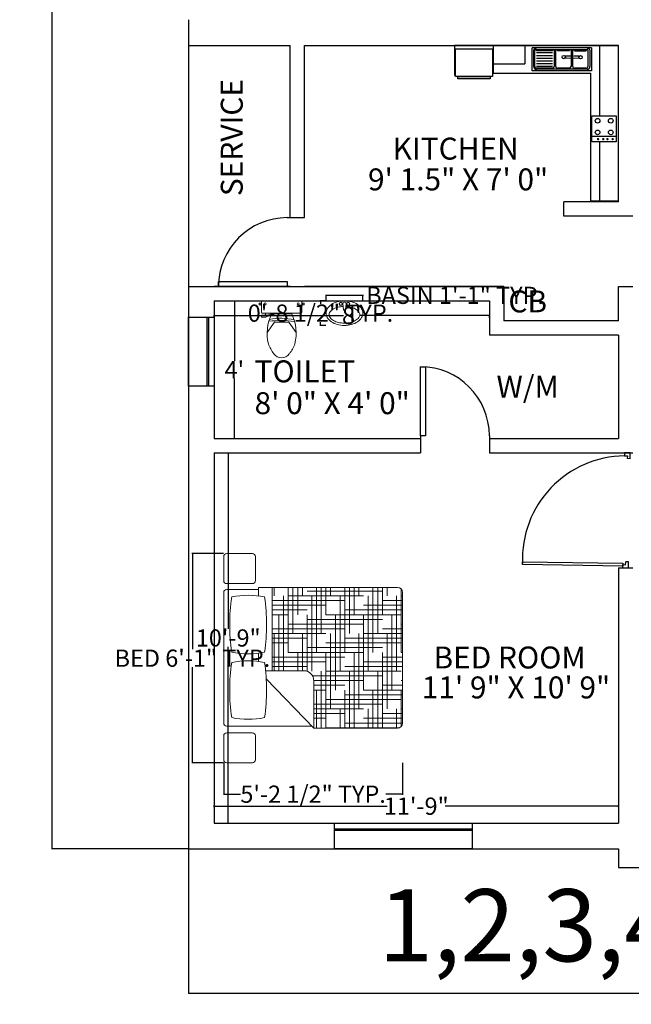
# Model space of a CAD drawing. Units: inches. Extents: x -113 to 5399, y -1393 to 3302.
# Tile 11 of 40: x 1545 to 1759, y 82 to 426. Entities that reach past the tile are written whole.
import ezdxf

# ---------------------------------------------------------------- set-up
doc = ezdxf.new("R2010")
doc.units = ezdxf.units.IN
doc.header["$MEASUREMENT"] = 0
for name, color, linetype, lineweight in [('A-ANNO-DIMS', 254, 'Continuous', 18), ('A-ANNO-TEXT', 7, 'Continuous', 25), ('A-AREA-IDEN', 4, 'Continuous', 18), ('A-FLOR-CASE', 8, 'Continuous', 18), ('A-FLOR-FIXT', 8, 'Continuous', 18), ('doors', 2, 'Continuous', 25), ('DT TEXT', 4, 'Continuous', 18), ('furniture', 131, 'Continuous', 18), ('walls', 1, 'Continuous', 25), ('windows', 3, 'Continuous', 25)]:
    doc.layers.add(name, color=color, linetype=linetype, lineweight=lineweight)
doc.layers.add('A-GLAZ-PATT', color=85, linetype='Continuous', lineweight=13, true_color=0x58ba48)
doc.layers.add('TEFRIŞ', color=11, linetype='Continuous')
doc.styles.get("Standard").update_dxf_attribs({"font": 'arial.ttf'})
doc.dimstyles.get("Standard").update_dxf_attribs({"dimtxt": 6, "dimasz": 0.18, "dimexe": 0.18, "dimexo": 0.0625, "dimgap": 0.09, "dimtad": 0, "dimtih": 1, "dimtoh": 1, "dimdec": 1, "dimzin": 0, "dimdsep": 46, "dimlunit": 4, "dimtxsty": 'Standard', "dimblk": 'ARCHTICK', "dimcen": 0.09, "dimadec": 0, "dimazin": 0, "dimtfac": 1, "dimtdec": 1, "dimtofl": 0, "dimtmove": 0, "dimatfit": 3, "dimfxl": 1, "dimtolj": 1, "dimtzin": 0, "dimarcsym": 0})

# ---------------------------------------------------------------- blocks, each defined once
blk = doc.blocks.new('*U2')
for p, q in [((0, 0), (0, -6)), ((24, 0), (24, -6))]:
    blk.add_line(p, q)
blk.add_lwpolyline([(0, 0), (0, 24), (1.75, 24), (1.75, 0)], close=True)
blk.add_arc((0, 0), 24, 0, 90)
blk = doc.blocks.new('*X4')
at = {"color": 0}
for p, q in [((4.3594, 18.5625), (4.3594, 18.6457)), ((4.5, 18), (4.5, 18.6457)), ((4.5469, 18.1875), (4.5469, 18.6457)), ((4.5938, 18.375), (4.5938, 18.6457)), ((4.6406, 18.5625), (4.6406, 18.6457)), ((4.7812, 18), (4.7812, 18.6457)), ((4.8281, 18.1875), (4.8281, 18.6457)), ((4.875, 18.375), (4.875, 18.6457)), ((4.9219, 18.5625), (4.9219, 18.6457)), ((5.0625, 18), (5.0625, 18.6457)), ((5.1094, 18.1875), (5.1094, 18.6457)), ((5.1562, 18.375), (5.1562, 18.6457)), ((5.2031, 18.5625), (5.2031, 18.6457)), ((5.3438, 18), (5.3438, 18.6457)), ((5.3906, 18.1875), (5.3906, 18.6457)), ((5.4375, 18.375), (5.4375, 18.6457)), ((5.4844, 18.5625), (5.4844, 18.6457)), ((5.625, 18), (5.625, 18.6287)), ((4.4531, 17.8169), (4.4531, 18.5625)), ((4.5, 18.5625), (5.25, 18.5625)), ((4.6875, 18.6094), (5.4375, 18.6094)), ((4.7344, 17.8125), (4.7344, 18.5625)), ((5.0156, 17.8125), (5.0156, 18.5625)), ((5.2969, 17.8125), (5.2969, 18.5625)), ((5.5781, 17.8125), (5.5781, 18.5625)), ((5.625, 18.5625), (5.6375, 18.5625)), ((4.3395, 18.5156), (5.0625, 18.5156)), ((4.3395, 18.4688), (4.875, 18.4688)), ((5.25, 18.4688), (5.6375, 18.4688)), ((5.4375, 18.5156), (5.6375, 18.5156)), ((4.3395, 18.4219), (4.6875, 18.4219)), ((4.3395, 18.375), (4.5, 18.375)), ((4.4062, 17.8169), (4.4062, 18.375)), ((4.6875, 17.8114), (4.6875, 18.375)), ((4.6875, 18.3281), (5.4375, 18.3281)), ((4.875, 18.375), (5.625, 18.375)), ((4.9688, 17.625), (4.9688, 18.375)), ((5.0625, 18.4219), (5.6375, 18.4219)), ((5.25, 17.625), (5.25, 18.375)), ((5.5312, 17.625), (5.5312, 18.375)), ((4.3395, 18.2344), (5.0625, 18.2344)), ((4.5, 18.2812), (5.25, 18.2812)), ((5.4375, 18.2344), (5.6375, 18.2344)), ((5.625, 18.2812), (5.6375, 18.2812)), ((4.3395, 18.1875), (4.875, 18.1875)), ((4.3395, 18.1406), (4.6875, 18.1406)), ((4.3594, 17.8169), (4.3594, 18.1875)), ((4.6406, 17.8169), (4.6406, 18.1875)), ((4.9219, 17.4375), (4.9219, 18.1875)), ((5.0625, 18.1406), (5.6375, 18.1406)), ((5.2031, 17.4375), (5.2031, 18.1875)), ((5.25, 18.1875), (5.6375, 18.1875)), ((5.4844, 17.4375), (5.4844, 18.1875)), ((4.3395, 18.0938), (4.5, 18.0938)), ((4.6875, 18.0469), (5.4375, 18.0469)), ((4.875, 18.0938), (5.625, 18.0938)), ((4.3395, 17.9531), (5.0625, 17.9531)), ((4.5, 18), (5.25, 18)), ((4.5938, 17.8169), (4.5938, 18)), ((4.875, 17.25), (4.875, 18)), ((5.1562, 17.25), (5.1562, 18)), ((5.4375, 17.25), (5.4375, 18)), ((5.4375, 17.9531), (5.6375, 17.9531)), ((5.625, 18), (5.6375, 18)), ((4.3395, 17.9062), (4.875, 17.9062)), ((4.3395, 17.8594), (4.6875, 17.8594)), ((5.0625, 17.8594), (5.6375, 17.8594)), ((5.25, 17.9062), (5.6375, 17.9062)), ((4.7421, 17.7656), (5.4375, 17.7656)), ((4.8281, 17.2457), (4.8281, 17.8125)), ((4.875, 17.8125), (5.625, 17.8125)), ((5.1094, 17.2457), (5.1094, 17.8125)), ((5.3906, 17.2457), (5.3906, 17.8125)), ((4.7548, 17.7188), (5.25, 17.7188)), ((4.7548, 17.6719), (5.0625, 17.6719)), ((5.4375, 17.6719), (5.6375, 17.6719)), ((5.625, 17.7188), (5.6375, 17.7188)), ((4.7548, 17.625), (4.875, 17.625)), ((4.7812, 17.2457), (4.7812, 17.625)), ((5.0625, 17.2457), (5.0625, 17.625)), ((5.0625, 17.5781), (5.6375, 17.5781)), ((5.25, 17.625), (5.6375, 17.625)), ((5.3438, 17.2457), (5.3438, 17.625)), ((5.625, 17.2627), (5.625, 17.625)), ((4.7548, 17.4844), (5.4375, 17.4844)), ((4.875, 17.5312), (5.625, 17.5312)), ((4.7548, 17.4375), (5.25, 17.4375)), ((4.7548, 17.3906), (5.0625, 17.3906)), ((5.0156, 17.2457), (5.0156, 17.4375)), ((5.2969, 17.2457), (5.2969, 17.4375)), ((5.4375, 17.3906), (5.6375, 17.3906)), ((5.5781, 17.2457), (5.5781, 17.4375)), ((5.625, 17.4375), (5.6375, 17.4375)), ((4.7548, 17.3438), (4.875, 17.3438)), ((4.875, 17.25), (5.6077, 17.25)), ((4.9688, 17.2457), (4.9688, 17.25)), ((5.0625, 17.2969), (5.6375, 17.2969)), ((5.25, 17.3438), (5.6375, 17.3438)), ((5.25, 17.2457), (5.25, 17.25)), ((5.5312, 17.2457), (5.5312, 17.25))]:
    blk.add_line(p, q, dxfattribs=at)
blk = doc.blocks.new('MAT-P01')
for p, q in [((-0.0213, 0.8164), (-0.0213, 0.5605)), ((0.0087, 0.8464), (0.2471, 0.8464)), ((0.2771, 0.8164), (0.2771, 0.5605)), ((0.3437, 0.8164), (0.3437, -0.0316)), ((0.3737, 0.8464), (1.6737, 0.8464)), ((1.7037, 0.8164), (1.7037, 0.5005)), ((1.7622, 0.8164), (1.7622, 0.5605)), ((1.7922, 0.8464), (2.0306, 0.8464)), ((2.0606, 0.8164), (2.0606, 0.5605)), ((0.0087, 0.5305), (0.2471, 0.5305)), ((0.9879, 0.5005), (1.0693, 0.5005)), ((1.6393, 0.5005), (1.7237, 0.5005)), ((1.7237, 0.5005), (1.7237, -0.8836)), ((1.7922, 0.5305), (2.0306, 0.5305)), ((0.8146, 0.423), (0.3237, -0.0509)), ((0.8949, 0.4293), (0.8949, 0.0491)), ((0.8949, 0.3643), (1.7237, 0.3643)), ((0.8949, 0.3643), (0.8949, 0.0491)), ((0.8949, 0.3643), (1.7237, 0.3643)), ((1.7237, 0.3643), (1.7237, -0.8836)), ((0.3237, -0.0509), (0.7949, -0.0509)), ((0.3237, -0.0509), (0.3237, -0.8836)), ((0.3737, -0.9336), (1.6737, -0.9336))]:
    blk.add_line(p, q)
for centre, radius, start, end in [((0.0087, 0.8164), 0.03, 90, 180), ((0.2471, 0.8164), 0.03, 0, 90), ((0.3737, 0.8164), 0.03, 90, 180), ((0.7029, -1.1436), 1.9306, 81.81622, 98.18378), ((1.3543, -1.1436), 1.9306, 81.81622, 98.18378), ((1.6737, 0.8164), 0.03, 0, 90), ((1.7922, 0.8164), 0.03, 90, 180), ((2.0306, 0.8164), 0.03, 0, 90), ((1.2251, 0.6034), 0.8138, 168.37298, 191.62702), ((0.1806, 0.6034), 0.8138, 348.37298, 11.62702), ((1.8766, 0.6034), 0.8138, 168.37298, 191.62702), ((0.8321, 0.6034), 0.8138, 348.37298, 11.62702), ((0.0087, 0.5605), 0.03, 180, 270), ((0.2471, 0.5605), 0.03, 270, 0), ((1.7922, 0.5605), 0.03, 180, 270), ((2.0306, 0.5605), 0.03, 270, 0), ((0.7029, 2.3504), 1.9306, 261.81622, 278.18378), ((1.3543, 2.3504), 1.9306, 261.81622, 278.18378), ((0.7949, 0.0491), 0.1, 270, 0), ((0.3737, -0.8836), 0.05, 180, 270), ((1.6737, -0.8836), 0.05, 270, 0)]:
    blk.add_arc(centre, radius, start, end)
at = {"rotation": 270}
blk.add_blockref('*X4', (-16.9221, 4.7038), dxfattribs=at)
blk = doc.blocks.new('A$C008029BD')
at = {"layer": 'TEFRIŞ', "ltscale": 0.05}
for p, q in [((0, 0), (0, -3.55)), ((3.37, 0), (0, 0)), ((3.37, 0), (3.37, -0.6)), ((1.522, -0.4), (0, -0.4)), ((3.37, -0.4), (2.083, -0.4)), ((0.05, -0.581), (0.05, -1.869)), ((0.05, -0.581), (0.55, -0.581)), ((0.096, -0.617), (0.454, -0.617)), ((0.55, -0.581), (0.55, -1.869)), ((0.6, -2.71), (0.6, -0.6)), ((3.37, -0.6), (0.6, -0.6)), ((0.086, -1.773), (0.086, -0.677)), ((0.099, -0.659), (0.457, -0.659)), ((0.113, -0.954), (0.113, -0.695)), ((0.23, -0.846), (0.229, -0.967)), ((0.28, -0.846), (0.277, -1.158)), ((0.493, -0.695), (0.493, -0.954)), ((0.514, -0.677), (0.514, -1.773)), ((0.096, -1.024), (0.454, -1.024)), ((0.457, -0.99), (0.099, -0.99)), ((0.11, -1.319), (0.11, -1.06)), ((0.228, -1.02), (0.227, -1.159)), ((0.49, -1.06), (0.49, -1.319)), ((0.454, -1.355), (0.096, -1.355)), ((0.096, -1.391), (0.454, -1.391)), ((0.11, -1.773), (0.11, -1.427)), ((0.154, -1.773), (0.154, -1.427)), ((0.214, -1.773), (0.214, -1.427)), ((0.274, -1.773), (0.274, -1.427)), ((0.334, -1.773), (0.334, -1.427)), ((0.39, -1.773), (0.39, -1.427)), ((0.444, -1.773), (0.444, -1.427)), ((0.49, -1.427), (0.49, -1.773)), ((0.55, -1.869), (0.05, -1.869)), ((0.454, -1.809), (0.096, -1.809)), ((0.454, -1.833), (0.096, -1.833)), ((0, -2.025), (0.4, -2.025)), ((0.4, -2.71), (0.4, -2.025)), ((0, -2.71), (0.6, -2.71)), ((0, -3.55), (0.65, -3.55))]:
    blk.add_line(p, q, dxfattribs=at)
at = {"layer": 'TEFRIŞ'}
blk.add_line((1.969, -0.05), (1.969, -0.572), dxfattribs=at)
at = {"layer": 'TEFRIŞ', "ltscale": 0.05}
for points in [[(1.522, -0.05), (2.083, -0.05), (2.083, -0.572), (1.522, -0.572)], [(0.67, -2.73), (0.67, -3.53), (0.07, -3.53), (0.07, -2.73)], [(0.72, -2.78), (0.72, -3.48), (0.67, -3.48), (0.67, -2.78)]]:
    blk.add_lwpolyline(points, close=True, dxfattribs=at)
at = {"layer": 'TEFRIŞ', "const_width": 0.025}
for points in [[(2.014, -0.123, 1), (2.039, -0.123, 1)], [(2.014, -0.236, 1), (2.039, -0.236, 1)], [(2.014, -0.327, 1), (2.039, -0.327, 1)], [(2.014, -0.44, 1), (2.039, -0.44, 1)]]:
    blk.add_lwpolyline(points, format="xyb", close=True, dxfattribs=at)
at = {"layer": 'TEFRIŞ', "ltscale": 0.05}
for centre, radius in [((1.628, -0.164), 0.0505), ((1.628, -0.45), 0.0505), ((0.255, -0.82), 0.036), ((0.252, -1.184), 0.036)]:
    blk.add_circle(centre, radius, dxfattribs=at)
at = {"layer": 'TEFRIŞ'}
for centre in [(1.88, -0.164), (1.88, -0.45)]:
    blk.add_circle(centre, 0.0505, dxfattribs=at)
at = {"layer": 'TEFRIŞ', "ltscale": 0.05}
for centre, radius, start, end in [((0.108, -0.649), 0.0351, 110.4976, 230.5777), ((0.454, -0.677), 0.06, 0, 90), ((0.118, -0.673), 0.023, 143.9853, 258.5157), ((0.457, -0.695), 0.036, 0, 90), ((0.115, -1.038), 0.023, 143.9853, 258.5157), ((0.118, -0.976), 0.023, 101.4843, 216.0147), ((0.454, -1.06), 0.036, 0, 90), ((0.457, -0.954), 0.036, 270, 0), ((0.115, -1.341), 0.023, 101.4843, 216.0147), ((0.115, -1.405), 0.023, 143.9853, 258.5157), ((0.454, -1.319), 0.036, 270, 0), ((0.454, -1.427), 0.036, 0, 90), ((0.108, -1.801), 0.0351, 129.4223, 249.5024), ((0.115, -1.796), 0.023, 101.4843, 216.0147), ((0.454, -1.773), 0.06, 270, 0), ((0.454, -1.773), 0.036, 270, 0)]:
    blk.add_arc(centre, radius, start, end, dxfattribs=at)
blk = doc.blocks.new('toilet-3')
at = {"color": 0, "linetype": 'ByBlock'}
for p, q in [((-0.281, -0.05), (-0.281, -0.069)), ((-0.281, -0.05), (-0.261, -0.05)), ((-0.281, -0.069), (-0.261, -0.069)), ((-0.261, -0.047), (-0.261, -0.072)), ((-0.261, -0.047), (-0.251, -0.047)), ((-0.261, -0.072), (-0.251, -0.072)), ((-0.251, -0.047), (-0.251, -0.072)), ((-0.25, -0.03), (-0.25, -0.165)), ((0.24, -0.02), (-0.24, -0.02)), ((0.25, -0.03), (0.25, -0.165)), ((0.261, -0.047), (0.251, -0.047)), ((0.251, -0.047), (0.251, -0.072)), ((0.261, -0.072), (0.251, -0.072)), ((0.261, -0.047), (0.261, -0.072)), ((0.281, -0.05), (0.261, -0.05)), ((0.281, -0.069), (0.261, -0.069)), ((0.281, -0.05), (0.281, -0.069)), ((-0.144, -0.2), (-0.25, -0.2)), ((-0.25, -0.2), (-0.25, -0.222)), ((-0.198, -0.222), (-0.25, -0.222)), ((0.24, -0.175), (-0.24, -0.175)), ((-0.202, -0.2), (-0.202, -0.175)), ((-0.198, -0.222), (-0.16, -0.207)), ((-0.16, -0.207), (-0.16, -0.2)), ((-0.144, -0.2), (-0.144, -0.175)), ((0.125, -0.182), (-0.125, -0.182)), ((-0.089, -0.287), (-0.18, -0.415)), ((0.089, -0.287), (-0.089, -0.287)), ((0.089, -0.287), (0.18, -0.415))]:
    blk.add_line(p, q, dxfattribs=at)
for centre in [(-0.205, -0.059), (0.205, -0.059)]:
    blk.add_circle(centre, 0.0125, dxfattribs=at)
for centre, radius, start, end in [((-0.24, -0.03), 0.01, 90, 180), ((0.24, -0.03), 0.01, 0, 90), ((-0.24, -0.165), 0.01, 180, 270), ((0.376, -0.424), 0.557, 154.2321, 193.6755), ((-0.005, -0.896), 0.659, 75.9276, 103.0204), ((-0.376, -0.424), 0.557, 346.3245, 25.7679), ((0.24, -0.165), 0.01, 270, 0), ((-0.013, -1.787), 1.521, 83.4552, 95.5271), ((0.262, -0.406), 0.452, 199.2942, 217.2549), ((-0.265, -0.4), 0.457, 322.2382, 340.1051), ((-0.001, -0.609), 0.12, 216.3794, 323.6206)]:
    blk.add_arc(centre, radius, start, end, dxfattribs=at)
blk = doc.blocks.new('wash-6')
at = {"color": 0, "linetype": 'ByBlock'}
for p, q in [((-0.036, -0.063), (-0.021, -0.18)), ((0.036, -0.063), (0.021, -0.18))]:
    blk.add_line(p, q, dxfattribs=at)
for centre, radius in [((-0.075, -0.062), 0.0325), ((-0.075, -0.062), 0.0263), ((0.075, -0.062), 0.0325), ((0.075, -0.062), 0.0263)]:
    blk.add_circle(centre, radius, dxfattribs=at)
for centre, radius, start, end in [((0, -0.56), 0.56, 90, 105.4371), ((-0.204, -0.25), 0.17, 148.1465, 180), ((-0.107, -0.311), 0.285, 123.6901, 148.1465), ((-0.114, -0.361), 0.225, 118.369, 142.5096), ((-0.042, -0.407), 0.401, 105.4371, 123.6901), ((-0.045, -0.488), 0.37, 102.6081, 118.369), ((0, -0.69), 0.576, 92.9466, 102.6081), ((0, -0.063), 0.0361, 0, 180), ((0, -0.18), 0.0215, 180, 0), ((0, -0.56), 0.56, 74.5629, 90), ((0, -0.69), 0.576, 77.3919, 87.0534), ((0.045, -0.488), 0.37, 61.631, 77.3919), ((0.042, -0.407), 0.401, 56.3099, 74.5629), ((0.114, -0.361), 0.225, 37.4904, 61.631), ((0.107, -0.311), 0.285, 31.8535, 56.3099), ((0.204, -0.25), 0.17, 0, 31.8535), ((-0.204, -0.25), 0.17, 180, 211.8535), ((-0.107, -0.189), 0.285, 211.8535, 236.3099), ((-0.217, -0.282), 0.0954, 142.5096, 180), ((-0.217, -0.282), 0.0954, 180, 217.4904), ((-0.114, -0.203), 0.225, 217.4904, 241.631), ((0.114, -0.203), 0.225, 298.369, 322.5096), ((0.107, -0.189), 0.285, 303.6901, 328.1465), ((0.217, -0.282), 0.0954, 0, 37.4904), ((0.217, -0.282), 0.0954, 322.5096, 0), ((0.204, -0.25), 0.17, 328.1465, 0), ((-0.042, -0.092), 0.401, 236.3099, 254.5629), ((-0.045, -0.076), 0.37, 241.631, 257.3919), ((0, 0.06), 0.56, 254.5629, 270), ((0, 0.125), 0.576, 257.3919, 270), ((0, 0.125), 0.576, 270, 282.6081), ((0, 0.06), 0.56, 270, 285.4371), ((0.045, -0.076), 0.37, 282.6081, 298.369), ((0.042, -0.092), 0.401, 285.4371, 303.6901)]:
    blk.add_arc(centre, radius, start, end, dxfattribs=at)
blk = doc.blocks.new('_ArchTick')
at = {"color": 0, "linetype": 'ByBlock', "const_width": 0.15}
blk.add_lwpolyline([(-0.5, -0.5), (0.5, 0.5)], dxfattribs=at)
blk = doc.blocks.new('*D59')
at = {"layer": 'A-ANNO-DIMS', "color": 0, "lineweight": -2, "transparency": 16777216}
for p, q in [((1604.26, 136.47), (1604.26, 86.09)), ((2037.26, 136.47), (2037.26, 86.09)), ((1604.26, 86.27), (1810.37, 86.27)), ((2037.26, 86.27), (1831.16, 86.27))]:
    blk.add_line(p, q, dxfattribs=at)
at = {"layer": 'Defpoints', "color": 0, "transparency": 16777216}
for p in [(1604.26, 136.53), (2037.26, 136.53), (2037.26, 86.27)]:
    blk.add_point(p, dxfattribs=at)
at = {"layer": 'A-ANNO-DIMS', "color": 0, "lineweight": -2, "transparency": 16777216, "xscale": 0.18, "yscale": 0.18, "zscale": 0.18, "rotation": 180}
blk.add_blockref('_ArchTick', (1604.26, 86.27), dxfattribs=at)
at = {"layer": 'A-ANNO-DIMS', "color": 0, "lineweight": -2, "transparency": 16777216, "xscale": 0.18, "yscale": 0.18, "zscale": 0.18}
blk.add_blockref('_ArchTick', (2037.26, 86.27), dxfattribs=at)
at = {"layer": 'A-ANNO-DIMS', "color": 0, "transparency": 16777216, "insert": (1820.76, 86.27), "char_height": 6, "attachment_point": 5}
blk.add_mtext('\\A1;36\'-1"', dxfattribs=at)
blk = doc.blocks.new('*D60')
at = {"layer": 'A-ANNO-DIMS', "color": 0, "lineweight": -2, "transparency": 16777216}
for p, q in [((1604.2, 786.53), (1556.55, 786.53)), ((1556.73, 786.53), (1556.73, 464.69)), ((1556.73, 136.53), (1556.73, 458.38)), ((1604.2, 136.53), (1556.55, 136.53))]:
    blk.add_line(p, q, dxfattribs=at)
at = {"layer": 'Defpoints', "color": 0, "transparency": 16777216}
for p in [(1604.26, 786.53), (1556.73, 136.53), (1604.26, 136.53)]:
    blk.add_point(p, dxfattribs=at)
at = {"layer": 'A-ANNO-DIMS', "color": 0, "lineweight": -2, "transparency": 16777216, "xscale": 0.18, "yscale": 0.18, "zscale": 0.18}
for p, rotation in [((1556.73, 786.53), 90), ((1556.73, 136.53), 270)]:
    blk.add_blockref('_ArchTick', p, dxfattribs=dict(at, rotation=rotation))
at = {"layer": 'A-ANNO-DIMS', "color": 0, "transparency": 16777216, "insert": (1556.73, 461.53), "char_height": 6, "attachment_point": 5}
blk.add_mtext('\\A1;54\'-2"', dxfattribs=at)
blk = doc.blocks.new('*D67')
at = {"layer": 'A-ANNO-DIMS', "color": 0, "lineweight": -2, "transparency": 16777216}
for p, q in [((1617.62, 274.53), (1618.35, 274.53)), ((1618.17, 274.53), (1618.17, 213.19)), ((1618.17, 145.53), (1618.17, 206.88)), ((1617.62, 145.53), (1618.35, 145.53))]:
    blk.add_line(p, q, dxfattribs=at)
at = {"layer": 'Defpoints', "color": 0, "transparency": 16777216}
for p in [(1617.55, 274.53), (1617.55, 145.53), (1618.17, 145.53)]:
    blk.add_point(p, dxfattribs=at)
at = {"layer": 'A-ANNO-DIMS', "color": 0, "lineweight": -2, "transparency": 16777216, "xscale": 0.18, "yscale": 0.18, "zscale": 0.18}
for p, rotation in [((1618.17, 274.53), 90), ((1618.17, 145.53), 270)]:
    blk.add_blockref('_ArchTick', p, dxfattribs=dict(at, rotation=rotation))
at = {"layer": 'A-ANNO-DIMS', "color": 0, "transparency": 16777216, "insert": (1618.17, 210.03), "char_height": 6, "attachment_point": 5}
blk.add_mtext('\\A1;10\'-9"', dxfattribs=at)
blk = doc.blocks.new('*D68')
at = {"layer": 'A-ANNO-DIMS', "color": 0, "lineweight": -2, "transparency": 16777216}
for p, q in [((1613.26, 151.05), (1613.26, 151.58)), ((1613.26, 151.4), (1673.65, 151.4)), ((1754.26, 151.4), (1693.88, 151.4)), ((1754.26, 151.05), (1754.26, 151.58))]:
    blk.add_line(p, q, dxfattribs=at)
at = {"layer": 'Defpoints', "color": 0, "transparency": 16777216}
for p in [(1754.26, 151.4), (1613.26, 150.98), (1754.26, 150.98)]:
    blk.add_point(p, dxfattribs=at)
at = {"layer": 'A-ANNO-DIMS', "color": 0, "lineweight": -2, "transparency": 16777216, "xscale": 0.18, "yscale": 0.18, "zscale": 0.18, "rotation": 180}
blk.add_blockref('_ArchTick', (1613.26, 151.4), dxfattribs=at)
at = {"layer": 'A-ANNO-DIMS', "color": 0, "lineweight": -2, "transparency": 16777216, "xscale": 0.18, "yscale": 0.18, "zscale": 0.18}
blk.add_blockref('_ArchTick', (1754.26, 151.4), dxfattribs=at)
at = {"layer": 'A-ANNO-DIMS', "color": 0, "transparency": 16777216, "insert": (1683.76, 151.4), "char_height": 6, "attachment_point": 5}
blk.add_mtext('\\A1;11\'-9"', dxfattribs=at)
blk = doc.blocks.new('*D77')
at = {"layer": 'A-ANNO-DIMS', "color": 0, "lineweight": -2, "transparency": 16777216}
for p, q in [((1620.3, 327.53), (1620.3, 306.62)), ((1620.36, 327.53), (1620.48, 327.53)), ((1620.3, 279.53), (1620.3, 300.44)), ((1620.36, 279.53), (1620.48, 279.53))]:
    blk.add_line(p, q, dxfattribs=at)
at = {"layer": 'Defpoints', "color": 0, "transparency": 16777216}
for p in [(1620.3, 327.53), (1620.3, 279.53), (1620.3, 279.53)]:
    blk.add_point(p, dxfattribs=at)
at = {"layer": 'A-ANNO-DIMS', "color": 0, "lineweight": -2, "transparency": 16777216, "xscale": 0.18, "yscale": 0.18, "zscale": 0.18}
for p, rotation in [((1620.3, 327.53), 90), ((1620.3, 279.53), 270)]:
    blk.add_blockref('_ArchTick', p, dxfattribs=dict(at, rotation=rotation))
at = {"layer": 'A-ANNO-DIMS', "color": 0, "transparency": 16777216, "insert": (1620.3, 303.53), "char_height": 6, "attachment_point": 5}
blk.add_mtext("\\A1;4'", dxfattribs=at)
blk = doc.blocks.new('*D78')
at = {"layer": 'A-ANNO-DIMS', "color": 0, "lineweight": -2, "transparency": 16777216}
for p, q in [((1613.26, 321.59), (1613.26, 322.56)), ((1613.26, 322.38), (1658.41, 322.38)), ((1709.26, 322.38), (1664.12, 322.38)), ((1709.26, 321.59), (1709.26, 322.56))]:
    blk.add_line(p, q, dxfattribs=at)
at = {"layer": 'Defpoints', "color": 0, "transparency": 16777216}
for p in [(1613.26, 322.38), (1613.26, 321.53), (1709.26, 321.53)]:
    blk.add_point(p, dxfattribs=at)
at = {"layer": 'A-ANNO-DIMS', "color": 0, "lineweight": -2, "transparency": 16777216, "xscale": 0.18, "yscale": 0.18, "zscale": 0.18, "rotation": 180}
blk.add_blockref('_ArchTick', (1613.26, 322.38), dxfattribs=at)
at = {"layer": 'A-ANNO-DIMS', "color": 0, "lineweight": -2, "transparency": 16777216, "xscale": 0.18, "yscale": 0.18, "zscale": 0.18}
blk.add_blockref('_ArchTick', (1709.26, 322.38), dxfattribs=at)
at = {"layer": 'A-ANNO-DIMS', "color": 0, "transparency": 16777216, "insert": (1661.26, 322.38), "char_height": 6, "attachment_point": 5}
blk.add_mtext("\\A1;8'", dxfattribs=at)
blk = doc.blocks.new('WIN-PLAN-48IN')
h = blk.add_hatch(color=256)
h.dxf.hatch_style = 1
h.paths.add_polyline_path([(48, 2.5), (0, 2.5), (0, 2), (48, 2)])
for p, q in [((0, 9), (48, 9)), ((0, 0), (0, 9)), ((48, 9), (48, 0)), ((48, 2.5), (0, 2.5)), ((48, 2), (0, 2)), ((48, 0), (0, 0))]:
    blk.add_line(p, q)
blk = doc.blocks.new('DOOR-SINGLE-36IN-PLAN')
for p, q in [((0.5, 2), (0.5, 36.98)), ((0.5, 36.98), (1.5, 36.98)), ((1.5, 36.98), (1.5, 2)), ((0, 2), (0, 0)), ((0, 2), (1.04, 2)), ((1.5, 2), (0.5, 2)), ((1.04, 2), (1.04, 0.98)), ((1.04, 0.98), (2, 0.98)), ((2, 0), (2, 0.98)), ((38.96, 0.98), (38, 0.98)), ((38, 0), (38, 0.98)), ((40, 2), (38.96, 2)), ((38.96, 2), (38.96, 0.98)), ((40, 0), (40, 2)), ((0, 0), (2, 0)), ((0, 0), (2, 0)), ((38, 0), (40, 0))]:
    blk.add_line(p, q)
blk.add_arc((2.94, 0.99), 36.04, 1.6003, 93.0893)
blk = doc.blocks.new('*D171')
at = {"layer": 'A-ANNO-DIMS', "color": 0, "lineweight": -2, "transparency": 16777216}
for p, q in [((1616.55, 239.43), (1605.49, 239.43)), ((1605.67, 239.43), (1605.67, 206.13)), ((1605.67, 166.52), (1605.67, 199.82)), ((1616.55, 166.52), (1605.49, 166.52))]:
    blk.add_line(p, q, dxfattribs=at)
at = {"layer": 'Defpoints', "color": 0, "transparency": 16777216}
for p in [(1605.67, 239.43), (1616.61, 239.43), (1616.61, 166.52)]:
    blk.add_point(p, dxfattribs=at)
at = {"layer": 'A-ANNO-DIMS', "color": 0, "lineweight": -2, "transparency": 16777216, "xscale": 0.18, "yscale": 0.18, "zscale": 0.18}
for p, rotation in [((1605.67, 239.43), 90), ((1605.67, 166.52), 270)]:
    blk.add_blockref('_ArchTick', p, dxfattribs=dict(at, rotation=rotation))
at = {"layer": 'A-ANNO-DIMS', "color": 0, "transparency": 16777216, "insert": (1605.67, 202.97), "char_height": 6, "attachment_point": 5}
blk.add_mtext('\\A1;BED 6\'-1" TYP.', dxfattribs=at)
blk = doc.blocks.new('*D172')
at = {"layer": 'A-ANNO-DIMS', "color": 0, "lineweight": -2, "transparency": 16777216}
for p, q in [((1616.61, 166.45), (1616.61, 155.4)), ((1678.95, 166.45), (1678.95, 155.4)), ((1616.61, 155.58), (1622.41, 155.58)), ((1678.95, 155.58), (1673.15, 155.58))]:
    blk.add_line(p, q, dxfattribs=at)
at = {"layer": 'Defpoints', "color": 0, "transparency": 16777216}
for p in [(1616.61, 166.52), (1678.95, 166.52), (1616.61, 155.58)]:
    blk.add_point(p, dxfattribs=at)
at = {"layer": 'A-ANNO-DIMS', "color": 0, "lineweight": -2, "transparency": 16777216, "xscale": 0.18, "yscale": 0.18, "zscale": 0.18, "rotation": 180}
blk.add_blockref('_ArchTick', (1616.61, 155.58), dxfattribs=at)
at = {"layer": 'A-ANNO-DIMS', "color": 0, "lineweight": -2, "transparency": 16777216, "xscale": 0.18, "yscale": 0.18, "zscale": 0.18}
blk.add_blockref('_ArchTick', (1678.95, 155.58), dxfattribs=at)
at = {"layer": 'A-ANNO-DIMS', "color": 0, "transparency": 16777216, "insert": (1647.78, 155.58), "char_height": 6, "attachment_point": 5}
blk.add_mtext('\\A1;5\'-2 1/2" TYP.', dxfattribs=at)
blk = doc.blocks.new('*D179')
at = {"layer": 'A-ANNO-DIMS', "color": 0, "lineweight": -2, "transparency": 16777216}
for p, q in [((1652.28, 327.59), (1652.28, 329.64)), ((1665.14, 327.59), (1665.14, 329.64)), ((1652.28, 329.46), (1665.14, 329.46)), ((1665.14, 329.46), (1665.32, 329.46))]:
    blk.add_line(p, q, dxfattribs=at)
at = {"layer": 'Defpoints', "color": 0, "transparency": 16777216}
for p in [(1652.28, 327.53), (1665.14, 329.46), (1665.14, 327.53)]:
    blk.add_point(p, dxfattribs=at)
at = {"layer": 'A-ANNO-DIMS', "color": 0, "lineweight": -2, "transparency": 16777216, "xscale": 0.18, "yscale": 0.18, "zscale": 0.18, "rotation": 180}
blk.add_blockref('_ArchTick', (1652.28, 329.46), dxfattribs=at)
at = {"layer": 'A-ANNO-DIMS', "color": 0, "lineweight": -2, "transparency": 16777216, "xscale": 0.18, "yscale": 0.18, "zscale": 0.18}
blk.add_blockref('_ArchTick', (1665.14, 329.46), dxfattribs=at)
at = {"layer": 'A-ANNO-DIMS', "color": 0, "transparency": 16777216, "insert": (1697.3, 329.46), "char_height": 6, "attachment_point": 5}
blk.add_mtext('\\A1;BASIN 1\'-1" TYP.', dxfattribs=at)
blk = doc.blocks.new('*D180')
at = {"layer": 'A-ANNO-DIMS', "color": 0, "lineweight": -2, "transparency": 16777216}
for p, q in [((1652.22, 327.53), (1650.17, 327.53)), ((1650.35, 327.53), (1650.35, 326.44)), ((1650.35, 318.96), (1650.35, 320.05)), ((1652.22, 318.96), (1650.17, 318.96))]:
    blk.add_line(p, q, dxfattribs=at)
at = {"layer": 'Defpoints', "color": 0, "transparency": 16777216}
for p in [(1650.35, 327.53), (1652.28, 327.53), (1652.28, 318.96)]:
    blk.add_point(p, dxfattribs=at)
at = {"layer": 'A-ANNO-DIMS', "color": 0, "lineweight": -2, "transparency": 16777216, "xscale": 0.18, "yscale": 0.18, "zscale": 0.18}
for p, rotation in [((1650.35, 327.53), 90), ((1650.35, 318.96), 270)]:
    blk.add_blockref('_ArchTick', p, dxfattribs=dict(at, rotation=rotation))
at = {"layer": 'A-ANNO-DIMS', "color": 0, "transparency": 16777216, "insert": (1650.35, 323.25), "char_height": 6, "attachment_point": 5}
blk.add_mtext('\\A1;0\'-8 1/2" TYP.', dxfattribs=at)
blk = doc.blocks.new('*D209')
at = {"layer": 'A-ANNO-DIMS', "color": 0, "lineweight": -2, "transparency": 16777216}
for p, q in [((1754.32, 798.03), (2074.39, 798.03)), ((2074.21, 798.03), (2074.21, 467.19)), ((2074.21, 130.03), (2074.21, 460.88)), ((1754.32, 130.03), (2074.39, 130.03))]:
    blk.add_line(p, q, dxfattribs=at)
at = {"layer": 'Defpoints', "color": 0, "transparency": 16777216}
for p in [(1754.26, 798.03), (2074.21, 798.03), (1754.26, 130.03)]:
    blk.add_point(p, dxfattribs=at)
at = {"layer": 'A-ANNO-DIMS', "color": 0, "lineweight": -2, "transparency": 16777216, "xscale": 0.18, "yscale": 0.18, "zscale": 0.18}
for p, rotation in [((2074.21, 798.03), 90), ((2074.21, 130.03), 270)]:
    blk.add_blockref('_ArchTick', p, dxfattribs=dict(at, rotation=rotation))
at = {"layer": 'A-ANNO-DIMS', "color": 0, "transparency": 16777216, "insert": (2074.21, 464.03), "char_height": 6, "attachment_point": 5}
blk.add_mtext('\\A1;55\'-8"', dxfattribs=at)

msp = doc.modelspace()

# ---------------------------------------------------------------- hatches: boundary and pattern name
at = {"layer": 'A-GLAZ-PATT'}
h = msp.add_hatch(color=256, dxfattribs=at)
h.dxf.hatch_style = 1
h.paths.add_polyline_path([(1610.76, 321.81), (1610.76, 297.81), (1611.26, 297.81), (1611.26, 321.81)])

# ---------------------------------------------------------------- linework, layer by layer
at = {"layer": 'walls'}
for p, q in [((1604.26, 425.53), (1604.26, 136.53)), ((1604.26, 416.53), (1639.76, 416.53)), ((1639.76, 356.53), (1639.76, 416.53)), ((1644.76, 356.53), (1644.76, 416.53)), ((1644.76, 416.53), (1754.26, 416.53)), ((1754.26, 362.03), (1754.26, 416.53)), ((1754.26, 362.03), (1735.26, 362.03)), ((1735.26, 357.03), (1735.26, 362.03)), ((1759.26, 357.03), (1735.26, 357.03)), ((1639.76, 356.53), (1644.76, 356.53)), ((1604.26, 332.53), (1639.76, 332.53)), ((1639.76, 332.53), (1613.26, 332.53)), ((1639.76, 332.53), (1644.76, 332.53)), ((1714.26, 332.53), (1644.76, 332.53)), ((1644.76, 332.53), (1714.26, 332.53)), ((1714.26, 332.53), (1714.26, 320.53)), ((1754.26, 320.53), (1754.26, 332.53)), ((1754.26, 332.53), (1759.26, 332.53)), ((1613.26, 327.53), (1613.26, 279.53)), ((1613.26, 327.53), (1709.26, 327.53)), ((1613.26, 327.53), (1709.26, 327.53)), ((1709.26, 327.53), (1709.26, 315.53)), ((1754.26, 320.53), (1714.26, 320.53)), ((1754.26, 315.53), (1709.26, 315.53)), ((1754.26, 315.53), (1754.26, 279.53)), ((1613.26, 279.53), (1685.26, 279.53)), ((1685.26, 279.53), (1685.26, 274.53)), ((1709.26, 280.53), (1709.26, 274.53)), ((1709.26, 279.53), (1754.26, 279.53)), ((1613.26, 274.53), (1613.26, 145.53)), ((1613.26, 274.53), (1685.26, 274.53)), ((1709.26, 274.53), (1754.26, 274.53)), ((1754.26, 274.53), (1759.26, 274.53)), ((1754.26, 234.53), (1754.26, 145.53)), ((1754.26, 234.53), (1759.26, 234.53)), ((1613.26, 145.53), (1754.26, 145.53)), ((1604.26, 136.53), (1754.26, 136.53)), ((1754.26, 136.53), (1754.26, 130.03)), ((1754.26, 130.03), (1759.26, 130.03))]:
    msp.add_line(p, q, dxfattribs=at)
at = {"layer": 'windows'}
for p, q in [((1604.26, 297.81), (1604.26, 321.81)), ((1604.26, 321.81), (1613.26, 321.81)), ((1610.76, 321.81), (1610.76, 297.81)), ((1611.26, 321.81), (1611.26, 297.81)), ((1613.26, 321.81), (1613.26, 297.81)), ((1613.26, 297.81), (1604.26, 297.81))]:
    msp.add_line(p, q, dxfattribs=at)

# ---------------------------------------------------------------- block references
at = {"layer": 'A-FLOR-CASE', "xscale": 16.09806929200166, "yscale": 16.09806929200166, "zscale": 16.09806929200166, "rotation": 270}
msp.add_blockref('A$C008029BD', (1754.26, 416.53), dxfattribs=at)
at = {"layer": 'A-FLOR-FIXT'}
for name, p, xscale, yscale, zscale in [('toilet-3', (1636.8, 328.09), 27.95492935005888, 27.95492935005888, 27.95492935005888), ('wash-6', (1658.71, 327.53), 17.16666334294967, 17.16666334294967, 17.16666334294967)]:
    msp.add_blockref(name, p, dxfattribs=dict(at, xscale=xscale, yscale=yscale, zscale=zscale))
at = {"layer": 'doors'}
for name, p, rotation in [('*U2', (1638.76, 332.53), 90.00000000000003), ('DOOR-SINGLE-36IN-PLAN', (1757.76, 234.52), 89.09244041659088)]:
    msp.add_blockref(name, p, dxfattribs=dict(at, rotation=rotation))
msp.add_blockref('*U2', (1685.26, 280.53), dxfattribs=at)
at = {"layer": 'furniture', "xscale": 35.02364872074636, "yscale": 35.02364872074636, "zscale": 35.02364872074636, "rotation": 90}
msp.add_blockref('MAT-P01', (1646.25, 167.26), dxfattribs=at)
at = {"layer": 'windows', "rotation": 180}
msp.add_blockref('WIN-PLAN-48IN', (1703.26, 145.53), dxfattribs=at)

# ---------------------------------------------------------------- texts
at = {"layer": 'A-ANNO-TEXT'}
msp.add_text('1,2,3,4 FLOORS', height=25.17, dxfattribs=at).set_placement((1670.55, 97.29))
at = {"layer": 'A-AREA-IDEN'}
msp.add_text('SERVICE', height=7.647, rotation=90, dxfattribs=at).set_placement((1623.22, 364.03))
for s, height, p in [('KITCHEN', 7.647, (1675.52, 376.77)), ('9\' 1.5" X 7\' 0"', 7.6473, (1666.92, 366.04)), ('TOILET', 7.647, (1627.35, 299.13)), ('8\' 0" X 4\' 0"', 7.6473, (1627.35, 288.04)), ('BED ROOM', 7.647, (1689.77, 199.39)), ('11\' 9" X 10\' 9"', 7.6473, (1685.66, 188.96))]:
    msp.add_text(s, height=height, dxfattribs=at).set_placement(p)
at = {"layer": 'DT TEXT'}
for s, p in [('CB', (1715.89, 323.51)), (' W/M', (1709.42, 293.76))]:
    msp.add_text(s, height=7.647, dxfattribs=at).set_placement(p)

# ---------------------------------------------------------------- dimensions: what is measured, and where the dimension line sits
at = {"layer": 'A-ANNO-DIMS'}
for base, p1, p2, override, picture, middle in [((2074.21, 798.03), (1754.26, 130.03), (1754.26, 798.03), {"dimdec": 1, "dimlfac": 1, "dimrnd": 0, "dimzin": 1, "dimdsep": 46, "dimlunit": 4, "dimfrac": 2}, '*D209', (2074.21, 464.03)), ((1556.73, 136.53), (1604.26, 786.53), (1604.26, 136.53), {"dimclrd": 0, "dimclre": 0, "dimclrt": 0}, '*D60', (1556.73, 461.53)), ((1620.3, 279.53), (1620.3, 327.53), (1620.3, 279.53), {"dimclrd": 0, "dimclre": 0, "dimclrt": 0}, '*D77', (1620.3, 303.53)), ((1618.17, 145.53), (1617.55, 274.53), (1617.55, 145.53), {"dimclrd": 0, "dimclre": 0, "dimclrt": 0}, '*D67', (1618.17, 210.03))]:
    dim = msp.add_linear_dim(base=base, p1=p1, p2=p2, angle=90, dimstyle='Standard', override=override, dxfattribs=at)
    dim.commit()
    dim.dimension.update_dxf_attribs({"geometry": picture, "text_midpoint": middle})
dim = msp.add_linear_dim(base=(1665.14, 329.46), p1=(1652.28, 327.53), p2=(1665.14, 327.53), text='BASIN <> TYP.', dimstyle='Standard', override={"dimdec": 1, "dimlfac": 1, "dimrnd": 0, "dimzin": 1, "dimdsep": 46, "dimlunit": 4, "dimfrac": 2}, dxfattribs=at)
dim.commit()
dim.dimension.update_dxf_attribs({"geometry": '*D179', "text_midpoint": (1697.3, 329.46)})
for base, p1, p2, angle, text, picture, middle in [((1650.35, 327.53), (1652.28, 318.96), (1652.28, 327.53), 90, '<> TYP.', '*D180', (1650.35, 323.25)), ((1605.67, 239.43), (1616.61, 166.52), (1616.61, 239.43), 90, 'BED <> TYP.', '*D171', (1605.67, 202.97)), ((1616.61, 155.58), (1678.95, 166.52), (1616.61, 166.52), 180, '<> TYP.', '*D172', (1647.78, 155.58))]:
    dim = msp.add_linear_dim(base=base, p1=p1, p2=p2, angle=angle, text=text, dimstyle='Standard', override={"dimdec": 1, "dimlfac": 1, "dimrnd": 0, "dimzin": 1, "dimdsep": 46, "dimlunit": 4, "dimfrac": 2}, dxfattribs=at)
    dim.commit()
    dim.dimension.update_dxf_attribs({"geometry": picture, "text_midpoint": middle})
for base, p1, p2, picture, middle in [((1613.26, 322.38), (1709.26, 321.53), (1613.26, 321.53), '*D78', (1661.26, 322.38)), ((1754.26, 151.4), (1613.26, 150.98), (1754.26, 150.98), '*D68', (1683.76, 151.4)), ((2037.26, 86.27), (1604.26, 136.53), (2037.26, 136.53), '*D59', (1820.76, 86.27))]:
    dim = msp.add_linear_dim(base=base, p1=p1, p2=p2, dimstyle='Standard', override={"dimclrd": 0, "dimclre": 0, "dimclrt": 0}, dxfattribs=at)
    dim.commit()
    dim.dimension.update_dxf_attribs({"geometry": picture, "text_midpoint": middle})

doc.saveas('drawing.dxf')
